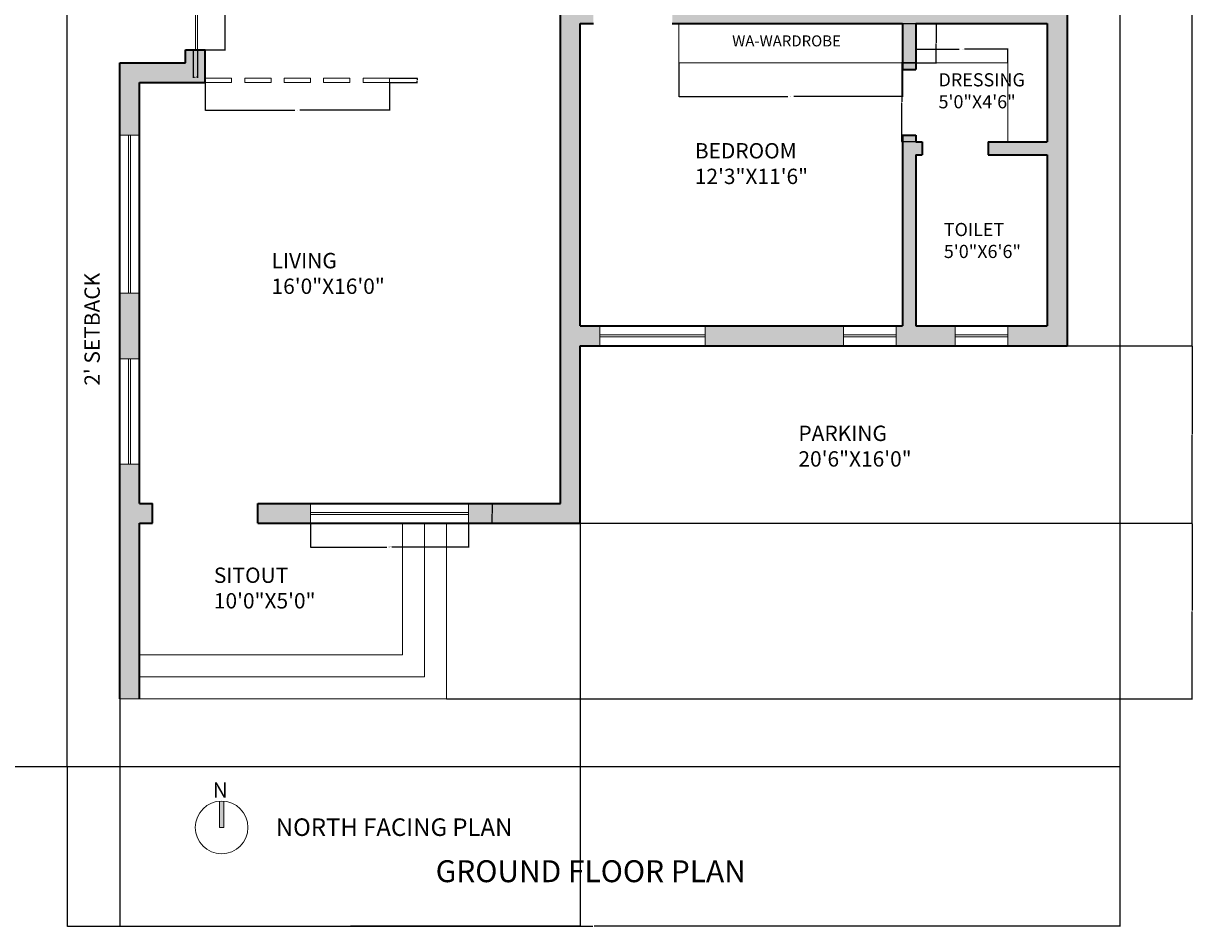
# Model space of a CAD drawing. Units: inches. Extents: x 3386 to 4477, y 1118 to 1824.
# Tile 6 of 7: x 3944 to 4477, y 1118 to 1530. Entities that reach past the tile are written whole.
import ezdxf

# ---------------------------------------------------------------- set-up
doc = ezdxf.new("R2010")
doc.units = ezdxf.units.IN
for name, color, linetype, lineweight in [('A-ANNO-DIMS', 2, 'Continuous', 18), ('A-ANNO-SYMB', 7, 'Continuous', 18), ('A-ANNO-TEXT', 7, 'Continuous', 18), ('A-ANNO-TITL', 7, 'Continuous', 25), ('A-AREA-IDEN', 7, 'Continuous', 18), ('A-DOOR', 4, 'Continuous', 18), ('A-FLOR-CASE', 7, 'Continuous', 18), ('A-FLOR-SCRN', 7, 'Continuous', 18), ('A-FLOR-STRS', 7, 'Continuous', 18), ('A-GLAZ', 4, 'Continuous', 18), ('A-WALL', 7, 'Continuous', 35), ('C-PROP', 7, 'Continuous', 25)]:
    doc.layers.add(name, color=color, linetype=linetype, lineweight=lineweight)
doc.layers.add('A-WALL-PATT', color=18, linetype='Continuous', lineweight=13, true_color=0x000000)
doc.styles.get("Standard").update_dxf_attribs({"font": 'arial.ttf'})
doc.dimstyles.get("Standard").update_dxf_attribs({"dimtxt": 0.18, "dimasz": 0.18, "dimexe": 0.18, "dimexo": 0.0625, "dimgap": 0.09, "dimtad": 0, "dimtih": 1, "dimtoh": 1, "dimdec": 4, "dimzin": 0, "dimdsep": 46, "dimtxsty": 'Standard', "dimcen": 0.09, "dimadec": 0, "dimazin": 0, "dimtfac": 1, "dimtdec": 4, "dimtofl": 0, "dimtmove": 0, "dimatfit": 3, "dimfxl": 1, "dimtolj": 1, "dimtzin": 0, "dimarcsym": 0})

# ---------------------------------------------------------------- blocks, each defined once
blk = doc.blocks.new('WIN-24IN')
for p, q in [((0, 0), (0, 9)), ((24, 0), (24, 9)), ((0, 5), (24, 5)), ((0, 4), (24, 4))]:
    blk.add_line(p, q)
blk = doc.blocks.new('WIN-48IN')
for p, q in [((0, 48), (9, 48)), ((4, 0), (4, 48)), ((5, 0), (5, 48)), ((0, 0), (9, 0))]:
    blk.add_line(p, q)
blk = doc.blocks.new('WIN-72IN')
for p, q in [((0, 0), (0, 9)), ((72, 0), (72, 9)), ((0, 5), (72, 5)), ((0, 4), (72, 4))]:
    blk.add_line(p, q)
blk = doc.blocks.new('DOOR-SLIDING-84IN')
for p, q in [((0, 42), (0, 84)), ((1, 84), (1, 0)), ((1, 42), (0, 42)), ((1, 42), (2, 42)), ((2, 42), (2, 0))]:
    blk.add_line(p, q)
blk = doc.blocks.new('NORTH-ARROW')
at = {"transparency": 33554687}
h = blk.add_hatch(color=256, dxfattribs=at)
h.dxf.hatch_style = 1
h.paths.add_polyline_path([(1, 0), (-1, 0), (-1, 11.96, -0.020861), (0, 12, -0.020861), (1, 11.96)])
for p, q in [((-1, 12), (-1, 0)), ((1, 0), (1, 11.96)), ((-1, 0), (1, 0))]:
    blk.add_line(p, q)
blk.add_circle((0, 0), 12)
blk.add_text('N', height=6.9).set_placement((-4.02, 13.6))
blk = doc.blocks.new('SCREEN-LIVING-DINING')
for points in [[(0, 0), (12, 0), (12, 2), (0, 2)], [(18, 0), (30, 0), (30, 2), (18, 2)], [(36, 0), (48, 0), (48, 2), (36, 2)], [(54, 0), (66, 0), (66, 2), (54, 2)], [(72, 0), (84, 0), (84, 2), (72, 2)]]:
    blk.add_lwpolyline(points, close=True)
blk = doc.blocks.new('WARDROBE-102IN')
for q in [(0, 18), (102, 0)]:
    blk.add_line((0, 0), q)
blk = doc.blocks.new('DRESSING-UNIT-42X36')
for p, q in [((0, 36), (42, 36)), ((42, 36), (42, 0))]:
    blk.add_line(p, q)
blk = doc.blocks.new('*D47')
at = {"layer": 'A-ANNO-DIMS', "color": 0, "lineweight": -2, "transparency": 16777216}
for p, q in [((4074.71, 1301.81), (4074.71, 1290.89)), ((4146.71, 1301.81), (4146.71, 1290.89)), ((4074.89, 1291.07), (4109.59, 1291.07)), ((4146.53, 1291.07), (4111.83, 1291.07))]:
    blk.add_line(p, q, dxfattribs=at)
at = {"layer": 'A-ANNO-DIMS', "color": 0, "transparency": 16777216}
for points in [[(4074.89, 1291.1), (4074.89, 1291.04), (4074.71, 1291.07)], [(4146.53, 1291.1), (4146.53, 1291.04), (4146.71, 1291.07)]]:
    blk.add_solid(points, dxfattribs=at)
at = {"layer": 'Defpoints', "color": 0, "transparency": 16777216}
for p in [(4074.71, 1301.87), (4146.71, 1301.87), (4146.71, 1291.07)]:
    blk.add_point(p, dxfattribs=at)
at = {"layer": 'A-ANNO-DIMS', "color": 0, "transparency": 16777216, "insert": (4110.71, 1291.07), "char_height": 0.18, "attachment_point": 5}
blk.add_mtext('\\A1;WINDOW 72 TYP.', dxfattribs=at)
blk = doc.blocks.new('*D48')
at = {"layer": 'A-ANNO-DIMS', "color": 0, "lineweight": -2, "transparency": 16777216}
for p, q in [((4146.77, 1310.87), (4157.69, 1310.87)), ((4157.51, 1310.69), (4157.51, 1306.55)), ((4146.77, 1301.87), (4157.69, 1301.87)), ((4157.51, 1302.05), (4157.51, 1306.19))]:
    blk.add_line(p, q, dxfattribs=at)
at = {"layer": 'A-ANNO-DIMS', "color": 0, "transparency": 16777216}
for points in [[(4157.48, 1310.69), (4157.54, 1310.69), (4157.51, 1310.87)], [(4157.48, 1302.05), (4157.54, 1302.05), (4157.51, 1301.87)]]:
    blk.add_solid(points, dxfattribs=at)
at = {"layer": 'Defpoints', "color": 0, "transparency": 16777216}
for p in [(4146.71, 1310.87), (4157.51, 1310.87), (4146.71, 1301.87)]:
    blk.add_point(p, dxfattribs=at)
at = {"layer": 'A-ANNO-DIMS', "color": 0, "transparency": 16777216, "insert": (4157.51, 1306.37), "char_height": 0.18, "attachment_point": 5}
blk.add_mtext('\\A1;9 TYP.', dxfattribs=at)
blk = doc.blocks.new('*D51')
at = {"layer": 'A-ANNO-DIMS', "color": 0, "lineweight": -2, "transparency": 16777216}
for p, q in [((4023.27, 1601.87), (4035.99, 1601.87)), ((4035.81, 1601.69), (4035.81, 1560.05)), ((4035.81, 1518.05), (4035.81, 1559.68)), ((4023.27, 1517.87), (4035.99, 1517.87))]:
    blk.add_line(p, q, dxfattribs=at)
at = {"layer": 'A-ANNO-DIMS', "color": 0, "transparency": 16777216}
for points in [[(4035.78, 1601.69), (4035.84, 1601.69), (4035.81, 1601.87)], [(4035.78, 1518.05), (4035.84, 1518.05), (4035.81, 1517.87)]]:
    blk.add_solid(points, dxfattribs=at)
at = {"layer": 'Defpoints', "color": 0, "transparency": 16777216}
for p in [(4023.21, 1601.87), (4023.21, 1517.87), (4035.81, 1517.87)]:
    blk.add_point(p, dxfattribs=at)
at = {"layer": 'A-ANNO-DIMS', "color": 0, "transparency": 16777216, "insert": (4035.81, 1559.87), "char_height": 0.18, "attachment_point": 5}
blk.add_mtext('\\A1;SLIDER 84 TYP.', dxfattribs=at)
blk = doc.blocks.new('*D52')
at = {"layer": 'A-ANNO-DIMS', "color": 0, "lineweight": -2, "transparency": 16777216}
for p, q in [((4021.21, 1517.81), (4021.21, 1505.09)), ((4023.21, 1517.81), (4023.21, 1505.09)), ((4021.39, 1505.27), (4021.75, 1505.27)), ((4023.03, 1505.27), (4022.67, 1505.27))]:
    blk.add_line(p, q, dxfattribs=at)
at = {"layer": 'A-ANNO-DIMS', "color": 0, "transparency": 16777216}
for points in [[(4021.39, 1505.3), (4021.39, 1505.24), (4021.21, 1505.27)], [(4023.03, 1505.3), (4023.03, 1505.24), (4023.21, 1505.27)]]:
    blk.add_solid(points, dxfattribs=at)
at = {"layer": 'Defpoints', "color": 0, "transparency": 16777216}
for p in [(4021.21, 1517.87), (4023.21, 1517.87), (4021.21, 1505.27)]:
    blk.add_point(p, dxfattribs=at)
at = {"layer": 'A-ANNO-DIMS', "color": 0, "transparency": 16777216, "insert": (4022.21, 1505.27), "char_height": 0.18, "attachment_point": 5}
blk.add_mtext('\\A1;2 TYP.', dxfattribs=at)
blk = doc.blocks.new('*D53')
at = {"layer": 'A-ANNO-DIMS', "color": 0, "lineweight": -2, "transparency": 16777216}
for p, q in [((4026.71, 1502.81), (4026.71, 1490.09)), ((4110.71, 1502.81), (4110.71, 1490.09)), ((4026.89, 1490.27), (4067.62, 1490.27)), ((4110.53, 1490.27), (4069.8, 1490.27))]:
    blk.add_line(p, q, dxfattribs=at)
at = {"layer": 'A-ANNO-DIMS', "color": 0, "transparency": 16777216}
for points in [[(4026.89, 1490.3), (4026.89, 1490.24), (4026.71, 1490.27)], [(4110.53, 1490.3), (4110.53, 1490.24), (4110.71, 1490.27)]]:
    blk.add_solid(points, dxfattribs=at)
at = {"layer": 'Defpoints', "color": 0, "transparency": 16777216}
for p in [(4026.71, 1502.87), (4110.71, 1502.87), (4110.71, 1490.27)]:
    blk.add_point(p, dxfattribs=at)
at = {"layer": 'A-ANNO-DIMS', "color": 0, "transparency": 16777216, "insert": (4068.71, 1490.27), "char_height": 0.18, "attachment_point": 5}
blk.add_mtext('\\A1;SCREEN 84 TYP.', dxfattribs=at)
blk = doc.blocks.new('*D54')
at = {"layer": 'A-ANNO-DIMS', "color": 0, "lineweight": -2, "transparency": 16777216}
for p, q in [((4110.77, 1504.87), (4123.49, 1504.87)), ((4123.31, 1504.69), (4123.31, 1504.05)), ((4123.31, 1503.05), (4123.31, 1503.69)), ((4110.77, 1502.87), (4123.49, 1502.87))]:
    blk.add_line(p, q, dxfattribs=at)
at = {"layer": 'A-ANNO-DIMS', "color": 0, "transparency": 16777216}
for points in [[(4123.28, 1504.69), (4123.34, 1504.69), (4123.31, 1504.87)], [(4123.28, 1503.05), (4123.34, 1503.05), (4123.31, 1502.87)]]:
    blk.add_solid(points, dxfattribs=at)
at = {"layer": 'Defpoints', "color": 0, "transparency": 16777216}
for p in [(4110.71, 1504.87), (4123.31, 1504.87), (4110.71, 1502.87)]:
    blk.add_point(p, dxfattribs=at)
at = {"layer": 'A-ANNO-DIMS', "color": 0, "transparency": 16777216, "insert": (4123.31, 1503.87), "char_height": 0.18, "attachment_point": 5}
blk.add_mtext('\\A1;2 TYP.', dxfattribs=at)
blk = doc.blocks.new('*D55')
at = {"layer": 'A-ANNO-DIMS', "color": 0, "lineweight": -2, "transparency": 16777216}
for p, q in [((4242.71, 1511.81), (4242.71, 1496.39)), ((4344.71, 1511.81), (4344.71, 1496.39)), ((4242.89, 1496.57), (4292.33, 1496.57)), ((4344.53, 1496.57), (4295.09, 1496.57))]:
    blk.add_line(p, q, dxfattribs=at)
at = {"layer": 'A-ANNO-DIMS', "color": 0, "transparency": 16777216}
for points in [[(4242.89, 1496.6), (4242.89, 1496.54), (4242.71, 1496.57)], [(4344.53, 1496.6), (4344.53, 1496.54), (4344.71, 1496.57)]]:
    blk.add_solid(points, dxfattribs=at)
at = {"layer": 'Defpoints', "color": 0, "transparency": 16777216}
for p in [(4242.71, 1511.87), (4344.71, 1511.87), (4344.71, 1496.57)]:
    blk.add_point(p, dxfattribs=at)
at = {"layer": 'A-ANNO-DIMS', "color": 0, "transparency": 16777216, "insert": (4293.71, 1496.57), "char_height": 0.18, "attachment_point": 5}
blk.add_mtext('\\A1;WARDROBE 102 TYP.', dxfattribs=at)
blk = doc.blocks.new('*D56')
at = {"layer": 'A-ANNO-DIMS', "color": 0, "lineweight": -2, "transparency": 16777216}
for p, q in [((4344.77, 1529.87), (4360.19, 1529.87)), ((4360.01, 1529.69), (4360.01, 1521.05)), ((4360.01, 1512.05), (4360.01, 1520.69)), ((4344.77, 1511.87), (4360.19, 1511.87))]:
    blk.add_line(p, q, dxfattribs=at)
at = {"layer": 'A-ANNO-DIMS', "color": 0, "transparency": 16777216}
for points in [[(4359.98, 1529.69), (4360.04, 1529.69), (4360.01, 1529.87)], [(4359.98, 1512.05), (4360.04, 1512.05), (4360.01, 1511.87)]]:
    blk.add_solid(points, dxfattribs=at)
at = {"layer": 'Defpoints', "color": 0, "transparency": 16777216}
for p in [(4344.71, 1529.87), (4360.01, 1529.87), (4344.71, 1511.87)]:
    blk.add_point(p, dxfattribs=at)
at = {"layer": 'A-ANNO-DIMS', "color": 0, "transparency": 16777216, "insert": (4360.01, 1520.87), "char_height": 0.18, "attachment_point": 5}
blk.add_mtext('\\A1;18 TYP.', dxfattribs=at)
blk = doc.blocks.new('*D61')
at = {"layer": 'A-ANNO-DIMS', "color": 0, "lineweight": -2, "transparency": 16777216}
for p, q in [((4350.71, 1511.93), (4350.71, 1518.35)), ((4350.89, 1518.17), (4370.54, 1518.17)), ((4392.53, 1518.17), (4372.88, 1518.17)), ((4392.71, 1511.93), (4392.71, 1518.35))]:
    blk.add_line(p, q, dxfattribs=at)
at = {"layer": 'A-ANNO-DIMS', "color": 0, "transparency": 16777216}
for points in [[(4350.89, 1518.2), (4350.89, 1518.14), (4350.71, 1518.17)], [(4392.53, 1518.2), (4392.53, 1518.14), (4392.71, 1518.17)]]:
    blk.add_solid(points, dxfattribs=at)
at = {"layer": 'Defpoints', "color": 0, "transparency": 16777216}
for p in [(4392.71, 1518.17), (4350.71, 1511.87), (4392.71, 1511.87)]:
    blk.add_point(p, dxfattribs=at)
at = {"layer": 'A-ANNO-DIMS', "color": 0, "transparency": 16777216, "insert": (4371.71, 1518.17), "char_height": 0.18, "attachment_point": 5}
blk.add_mtext('\\A1;DRESSER 42 TYP.', dxfattribs=at)
blk = doc.blocks.new('*D62')
at = {"layer": 'A-ANNO-DIMS', "color": 0, "lineweight": -2, "transparency": 16777216}
for p, q in [((4350.65, 1511.87), (4344.23, 1511.87)), ((4344.41, 1511.69), (4344.41, 1494.05)), ((4344.41, 1476.05), (4344.41, 1493.69)), ((4350.65, 1475.87), (4344.23, 1475.87))]:
    blk.add_line(p, q, dxfattribs=at)
at = {"layer": 'A-ANNO-DIMS', "color": 0, "transparency": 16777216}
for points in [[(4344.38, 1511.69), (4344.44, 1511.69), (4344.41, 1511.87)], [(4344.38, 1476.05), (4344.44, 1476.05), (4344.41, 1475.87)]]:
    blk.add_solid(points, dxfattribs=at)
at = {"layer": 'Defpoints', "color": 0, "transparency": 16777216}
for p in [(4344.41, 1511.87), (4350.71, 1511.87), (4350.71, 1475.87)]:
    blk.add_point(p, dxfattribs=at)
at = {"layer": 'A-ANNO-DIMS', "color": 0, "transparency": 16777216, "insert": (4344.41, 1493.87), "char_height": 0.18, "attachment_point": 5}
blk.add_mtext('\\A1;36 TYP.', dxfattribs=at)
blk = doc.blocks.new('*D105')
at = {"layer": 'A-ANNO-DIMS', "color": 0, "lineweight": -2, "transparency": 16777216}
for p, q in [((3963.71, 1190.81), (3963.71, 1117.96)), ((4443.71, 1190.81), (4443.71, 1117.96)), ((3963.89, 1118.14), (4203.42, 1118.14)), ((4443.53, 1118.14), (4204, 1118.14))]:
    blk.add_line(p, q, dxfattribs=at)
at = {"layer": 'A-ANNO-DIMS', "color": 0, "transparency": 16777216}
for points in [[(3963.89, 1118.17), (3963.89, 1118.11), (3963.71, 1118.14)], [(4443.53, 1118.17), (4443.53, 1118.11), (4443.71, 1118.14)]]:
    blk.add_solid(points, dxfattribs=at)
at = {"layer": 'Defpoints', "color": 0, "transparency": 16777216}
for p in [(3963.71, 1190.87), (4443.71, 1190.87), (4443.71, 1118.14)]:
    blk.add_point(p, dxfattribs=at)
at = {"layer": 'A-ANNO-DIMS', "color": 0, "transparency": 16777216, "insert": (4203.71, 1118.14), "char_height": 0.18, "attachment_point": 5}
blk.add_mtext('\\A1;480', dxfattribs=at)
blk = doc.blocks.new('*D106')
at = {"layer": 'A-ANNO-DIMS', "color": 0, "lineweight": -2, "transparency": 16777216}
for p, q in [((3963.65, 1790.87), (3930.48, 1790.87)), ((3930.66, 1790.69), (3930.66, 1491.05)), ((3930.66, 1191.05), (3930.66, 1490.69)), ((3963.65, 1190.87), (3930.48, 1190.87))]:
    blk.add_line(p, q, dxfattribs=at)
at = {"layer": 'A-ANNO-DIMS', "color": 0, "transparency": 16777216}
for points in [[(3930.63, 1790.69), (3930.69, 1790.69), (3930.66, 1790.87)], [(3930.63, 1191.05), (3930.69, 1191.05), (3930.66, 1190.87)]]:
    blk.add_solid(points, dxfattribs=at)
at = {"layer": 'Defpoints', "color": 0, "transparency": 16777216}
for p in [(3930.66, 1790.87), (3963.71, 1790.87), (3963.71, 1190.87)]:
    blk.add_point(p, dxfattribs=at)
at = {"layer": 'A-ANNO-DIMS', "color": 0, "transparency": 16777216, "insert": (3930.66, 1490.87), "char_height": 0.18, "attachment_point": 5}
blk.add_mtext('\\A1;600', dxfattribs=at)
blk = doc.blocks.new('*D108')
at = {"layer": 'A-ANNO-DIMS', "color": 0, "lineweight": -2, "transparency": 16777216}
for p, q in [((4197.71, 1301.81), (4197.71, 1117.96)), ((3987.71, 1221.81), (3987.71, 1117.96)), ((3987.89, 1118.14), (4092.42, 1118.14)), ((4197.53, 1118.14), (4093, 1118.14))]:
    blk.add_line(p, q, dxfattribs=at)
at = {"layer": 'A-ANNO-DIMS', "color": 0, "transparency": 16777216}
for points in [[(3987.89, 1118.17), (3987.89, 1118.11), (3987.71, 1118.14)], [(4197.53, 1118.17), (4197.53, 1118.11), (4197.71, 1118.14)]]:
    blk.add_solid(points, dxfattribs=at)
at = {"layer": 'Defpoints', "color": 0, "transparency": 16777216}
for p in [(4197.71, 1301.87), (3987.71, 1221.87), (4197.71, 1118.14)]:
    blk.add_point(p, dxfattribs=at)
at = {"layer": 'A-ANNO-DIMS', "color": 0, "transparency": 16777216, "insert": (4092.71, 1118.14), "char_height": 0.18, "attachment_point": 5}
blk.add_mtext('\\A1;210', dxfattribs=at)
blk = doc.blocks.new('*D109')
at = {"layer": 'A-ANNO-DIMS', "color": 0, "lineweight": -2, "transparency": 16777216}
for p, q in [((4197.77, 1301.87), (4476.94, 1301.87)), ((4476.76, 1301.69), (4476.76, 1262.05)), ((4476.76, 1222.05), (4476.76, 1261.69)), ((4136.77, 1221.87), (4476.94, 1221.87))]:
    blk.add_line(p, q, dxfattribs=at)
at = {"layer": 'A-ANNO-DIMS', "color": 0, "transparency": 16777216}
for points in [[(4476.73, 1301.69), (4476.79, 1301.69), (4476.76, 1301.87)], [(4476.73, 1222.05), (4476.79, 1222.05), (4476.76, 1221.87)]]:
    blk.add_solid(points, dxfattribs=at)
at = {"layer": 'Defpoints', "color": 0, "transparency": 16777216}
for p in [(4197.71, 1301.87), (4476.76, 1301.87), (4136.71, 1221.87)]:
    blk.add_point(p, dxfattribs=at)
at = {"layer": 'A-ANNO-DIMS', "color": 0, "transparency": 16777216, "insert": (4476.76, 1261.87), "char_height": 0.18, "attachment_point": 5}
blk.add_mtext('\\A1;80', dxfattribs=at)
blk = doc.blocks.new('*D110')
at = {"layer": 'A-ANNO-DIMS', "color": 0, "lineweight": -2, "transparency": 16777216}
for p, q in [((4419.77, 1382.87), (4476.94, 1382.87)), ((4476.76, 1382.69), (4476.76, 1342.55)), ((4476.76, 1302.05), (4476.76, 1342.19)), ((4197.77, 1301.87), (4476.94, 1301.87))]:
    blk.add_line(p, q, dxfattribs=at)
at = {"layer": 'A-ANNO-DIMS', "color": 0, "transparency": 16777216}
for points in [[(4476.73, 1382.69), (4476.79, 1382.69), (4476.76, 1382.87)], [(4476.73, 1302.05), (4476.79, 1302.05), (4476.76, 1301.87)]]:
    blk.add_solid(points, dxfattribs=at)
at = {"layer": 'Defpoints', "color": 0, "transparency": 16777216}
for p in [(4419.71, 1382.87), (4476.76, 1382.87), (4197.71, 1301.87)]:
    blk.add_point(p, dxfattribs=at)
at = {"layer": 'A-ANNO-DIMS', "color": 0, "transparency": 16777216, "insert": (4476.76, 1342.37), "char_height": 0.18, "attachment_point": 5}
blk.add_mtext('\\A1;81', dxfattribs=at)
blk = doc.blocks.new('*D111')
at = {"layer": 'A-ANNO-DIMS', "color": 0, "lineweight": -2, "transparency": 16777216}
for p, q in [((4419.77, 1766.87), (4476.94, 1766.87)), ((4476.76, 1766.69), (4476.76, 1575.05)), ((4476.76, 1383.05), (4476.76, 1574.69)), ((4419.77, 1382.87), (4476.94, 1382.87))]:
    blk.add_line(p, q, dxfattribs=at)
at = {"layer": 'A-ANNO-DIMS', "color": 0, "transparency": 16777216}
for points in [[(4476.73, 1766.69), (4476.79, 1766.69), (4476.76, 1766.87)], [(4476.73, 1383.05), (4476.79, 1383.05), (4476.76, 1382.87)]]:
    blk.add_solid(points, dxfattribs=at)
at = {"layer": 'Defpoints', "color": 0, "transparency": 16777216}
for p in [(4419.71, 1766.87), (4476.76, 1766.87), (4419.71, 1382.87)]:
    blk.add_point(p, dxfattribs=at)
at = {"layer": 'A-ANNO-DIMS', "color": 0, "transparency": 16777216, "insert": (4476.76, 1574.87), "char_height": 0.18, "attachment_point": 5}
blk.add_mtext('\\A1;384', dxfattribs=at)

msp = doc.modelspace()

# ---------------------------------------------------------------- hatches: boundary and pattern name
at = {"layer": 'A-WALL-PATT'}
h = msp.add_hatch(color=256, dxfattribs=at)
h.dxf.hatch_style = 1
h.paths.add_polyline_path([(4131.71, 1766.87), (4131.71, 1745.87), (4125.71, 1745.87), (4125.71, 1736.87), (4131.71, 1736.87), (4131.71, 1712.87), (4140.71, 1712.87), (4140.71, 1757.87), (4188.71, 1757.87), (4188.71, 1679.87), (4140.71, 1679.87), (4140.71, 1682.87), (4131.71, 1682.87), (4131.71, 1607.87), (4146.71, 1607.87), (4146.71, 1613.87), (4140.71, 1613.87), (4140.71, 1673.87), (4188.71, 1673.87), (4188.71, 1613.87), (4182.71, 1613.87), (4182.71, 1607.87), (4269.71, 1607.87), (4269.71, 1613.87), (4266.71, 1613.87), (4266.71, 1634.87), (4260.71, 1634.87), (4260.71, 1613.87), (4194.71, 1613.87), (4194.71, 1673.87), (4227.71, 1673.87), (4227.71, 1679.87), (4194.71, 1679.87), (4194.71, 1757.87), (4215.71, 1757.87), (4215.71, 1766.87)])
h.paths.add_polyline_path([(3987.71, 1688.87), (3996.71, 1688.87), (3996.71, 1736.87), (4035.71, 1736.87), (4035.71, 1745.87), (3987.71, 1745.87)])
h.paths.add_polyline_path([(3996.71, 1616.87), (3996.71, 1640.87), (3987.71, 1640.87), (3987.71, 1607.87), (4017.71, 1607.87), (4017.71, 1601.87), (4026.71, 1601.87), (4026.71, 1616.87)])
h.paths.add_polyline_path([(3987.71, 1511.87), (3987.71, 1478.87), (3996.71, 1478.87), (3996.71, 1502.87), (4026.71, 1502.87), (4026.71, 1517.87), (4017.71, 1517.87), (4017.71, 1511.87)])
h.paths.add_polyline_path([(3996.71, 1406.87), (3987.71, 1406.87), (3987.71, 1376.87), (3996.71, 1376.87)])
h.paths.add_polyline_path([(3996.71, 1310.87), (3996.71, 1328.87), (3987.71, 1328.87), (3987.71, 1221.87), (3996.71, 1221.87), (3996.71, 1301.87), (4002.71, 1301.87), (4002.71, 1310.87)])
h.paths.add_polyline_path([(4050.71, 1310.87), (4050.71, 1301.87), (4074.71, 1301.87), (4074.71, 1310.87)])
h.paths.add_polyline_path([(4197.71, 1301.87), (4197.71, 1382.87), (4206.71, 1382.87), (4206.71, 1391.87), (4197.71, 1391.87), (4197.71, 1529.87), (4203.71, 1529.87), (4203.71, 1535.87), (4188.71, 1535.87), (4188.71, 1310.87), (4146.71, 1310.87), (4146.71, 1301.87)])
h.paths.add_polyline_path([(4254.71, 1391.87), (4254.71, 1382.87), (4317.71, 1382.87), (4317.71, 1391.87)], flags=17)
h.paths.add_polyline_path([(4350.71, 1469.87), (4353.71, 1469.87), (4353.71, 1475.87), (4350.71, 1475.87), (4350.71, 1478.87), (4344.71, 1478.87), (4344.71, 1391.87), (4341.71, 1391.87), (4341.71, 1382.87), (4368.71, 1382.87), (4368.71, 1391.87), (4350.71, 1391.87)], flags=17)
h.paths.add_polyline_path([(4419.71, 1547.87), (4410.71, 1547.87), (4410.71, 1535.87), (4239.71, 1535.87), (4239.71, 1529.87), (4344.71, 1529.87), (4344.71, 1508.87), (4350.71, 1508.87), (4350.71, 1529.87), (4410.71, 1529.87), (4410.71, 1475.87), (4383.71, 1475.87), (4383.71, 1469.87), (4410.71, 1469.87), (4410.71, 1391.87), (4392.71, 1391.87), (4392.71, 1382.87), (4419.71, 1382.87)])
h.paths.add_polyline_path([(4419.71, 1673.87), (4410.71, 1673.87), (4410.71, 1613.87), (4305.71, 1613.87), (4305.71, 1607.87), (4410.71, 1607.87), (4410.71, 1595.87), (4419.71, 1595.87)])
h.paths.add_polyline_path([(4410.71, 1733.87), (4419.71, 1733.87), (4419.71, 1766.87), (4398.71, 1766.87), (4398.71, 1757.87), (4410.71, 1757.87)])
h.paths.add_polyline_path([(4266.71, 1757.87), (4272.71, 1757.87), (4272.71, 1766.87), (4239.71, 1766.87), (4239.71, 1757.87), (4260.71, 1757.87), (4260.71, 1679.87), (4257.71, 1679.87), (4257.71, 1673.87), (4260.71, 1673.87), (4260.71, 1664.87), (4266.71, 1664.87)])
h.paths.add_polyline_path([(4350.71, 1757.87), (4350.71, 1766.87), (4320.71, 1766.87), (4320.71, 1757.87)])
h.paths.add_polyline_path([(4083.71, 1745.87), (4083.71, 1736.87), (4095.71, 1736.87), (4095.71, 1745.87)])

# ---------------------------------------------------------------- linework, layer by layer
at = {"layer": 'A-FLOR-STRS'}
for p, q in [((4116.71, 1241.87), (4116.71, 1301.87)), ((4126.71, 1231.87), (4126.71, 1301.87)), ((4136.71, 1221.87), (4136.71, 1301.87)), ((3996.71, 1241.87), (4116.71, 1241.87)), ((3996.71, 1231.87), (4126.71, 1231.87)), ((3987.71, 1221.87), (4136.71, 1221.87))]:
    msp.add_line(p, q, dxfattribs=at)
at = {"layer": 'A-WALL'}
for p, q in [((4419.71, 1766.87), (4419.71, 1382.87)), ((4188.71, 1310.87), (4188.71, 1535.87)), ((4197.71, 1391.87), (4197.71, 1529.87)), ((4197.71, 1529.87), (4203.71, 1529.87)), ((4239.71, 1529.87), (4344.71, 1529.87)), ((4344.71, 1529.87), (4344.71, 1508.87)), ((4350.71, 1529.87), (4350.71, 1508.87)), ((4350.71, 1529.87), (4410.71, 1529.87)), ((4410.71, 1529.87), (4410.71, 1475.87)), ((4017.71, 1511.87), (4017.71, 1517.87)), ((4017.71, 1517.87), (4026.71, 1517.87)), ((4026.71, 1502.87), (4026.71, 1517.87)), ((3987.71, 1221.87), (3987.71, 1511.87)), ((3987.71, 1511.87), (4017.71, 1511.87)), ((4344.71, 1508.87), (4350.71, 1508.87)), ((3996.71, 1502.87), (4026.71, 1502.87)), ((3996.71, 1310.87), (3996.71, 1502.87)), ((4344.71, 1478.87), (4344.71, 1391.87)), ((4344.71, 1478.87), (4350.71, 1478.87)), ((4350.71, 1478.87), (4350.71, 1475.87)), ((4350.71, 1475.87), (4353.71, 1475.87)), ((4353.71, 1475.87), (4353.71, 1469.87)), ((4383.71, 1475.87), (4383.71, 1469.87)), ((4383.71, 1475.87), (4410.71, 1475.87)), ((4350.71, 1469.87), (4350.71, 1391.87)), ((4350.71, 1469.87), (4353.71, 1469.87)), ((4383.71, 1469.87), (4410.71, 1469.87)), ((4410.71, 1469.87), (4410.71, 1391.87)), ((4197.71, 1391.87), (4344.71, 1391.87)), ((4350.71, 1391.87), (4410.71, 1391.87)), ((4197.71, 1301.87), (4197.71, 1382.87)), ((4197.71, 1382.87), (4419.71, 1382.87)), ((3996.71, 1310.87), (4002.71, 1310.87)), ((4002.71, 1301.87), (4002.71, 1310.87)), ((4050.71, 1310.87), (4188.71, 1310.87)), ((4050.71, 1301.87), (4050.71, 1310.87)), ((3996.71, 1301.87), (4002.71, 1301.87)), ((3996.71, 1221.87), (3996.71, 1301.87)), ((4050.71, 1301.87), (4197.71, 1301.87))]:
    msp.add_line(p, q, dxfattribs=at)
at = {"layer": 'C-PROP'}
msp.add_lwpolyline([(3963.71, 1790.87), (4443.71, 1790.87), (4443.71, 1190.87), (3963.71, 1190.87)], close=True, dxfattribs=at)

# ---------------------------------------------------------------- block references
at = {"layer": 'A-ANNO-SYMB'}
msp.add_blockref('NORTH-ARROW', (4034.19, 1163.19), dxfattribs=at)
at = {"layer": 'A-DOOR', "rotation": 180}
msp.add_blockref('DOOR-SLIDING-84IN', (4023.21, 1601.87), dxfattribs=at)
at = {"layer": 'A-FLOR-CASE'}
for name, p in [('WARDROBE-102IN', (4242.71, 1511.87)), ('DRESSING-UNIT-42X36', (4350.71, 1475.87))]:
    msp.add_blockref(name, p, dxfattribs=at)
at = {"layer": 'A-FLOR-SCRN'}
msp.add_blockref('SCREEN-LIVING-DINING', (4026.71, 1502.87), dxfattribs=at)
at = {"layer": 'A-GLAZ'}
for name, p, rotation in [('WIN-72IN', (3987.71, 1478.87), 270.0000000000004), ('WIN-48IN', (4206.71, 1391.87), 269.9999999999996), ('WIN-24IN', (4341.71, 1391.87), 180), ('WIN-48IN', (3996.71, 1376.87), 180)]:
    msp.add_blockref(name, p, dxfattribs=dict(at, rotation=rotation))
for name, p in [('WIN-24IN', (4368.71, 1382.87)), ('WIN-72IN', (4074.71, 1301.87))]:
    msp.add_blockref(name, p, dxfattribs=at)

# ---------------------------------------------------------------- texts
at = {"layer": 'A-ANNO-TEXT', "insert": (4267.01, 1524.38), "char_height": 5, "attachment_point": 1}
msp.add_mtext_dynamic_manual_height_columns('{\\fTimes New Roman|b0|i0|c0|p18;WA-WARDROBE}', width=79.5604, gutter_width=12.5, heights=[0], dxfattribs=at)
at = {"layer": 'A-ANNO-TEXT', "insert": (3971.64, 1364.63), "char_height": 7, "attachment_point": 1, "rotation": 90}
msp.add_mtext_dynamic_manual_height_columns("{\\fTimes New Roman|b0|i0|c0|p18;2' SETBACK}", width=79.5604, gutter_width=12.5, heights=[0], dxfattribs=at)
at = {"layer": 'A-ANNO-TITL', "attachment_point": 1}
for s, insert, char_height in [('{\\fTimes New Roman|b0|i0|c0|p18;NORTH FACING PLAN}', (4058.88, 1167.31), 8), ('{\\fTimes New Roman|b0|i0|c0|p18;GROUND FLOOR PLAN}', (4131.79, 1148.22), 10)]:
    msp.add_mtext_dynamic_manual_height_columns(s, width=196.2607, gutter_width=12.5, heights=[0], dxfattribs=dict(at, insert=insert, char_height=char_height))
at = {"layer": 'A-AREA-IDEN', "attachment_point": 1}
for s, insert, char_height in [('{\\fTimes New Roman|b0|i0|c0|p18;DRESSING\\P5\'0"X4\'6"}', (4361.1, 1507.13), 6), ('{\\fTimes New Roman|b0|i0|c0|p18;BEDROOM\\P12\'3"X11\'6"}', (4249.97, 1475.27), 7), ('{\\fTimes New Roman|b0|i0|c0|p18;TOILET\\P5\'0"X6\'6"}', (4363.52, 1438.86), 6), ('{\\fTimes New Roman|b0|i0|c0|p18;LIVING\\P16\'0"X16\'0"}', (4056.95, 1425.17), 7), ('{\\fTimes New Roman|b0|i0|c0|p18;PARKING\\P20\'6"X16\'0"}', (4297.2, 1346.42), 7), ('{\\fTimes New Roman|b0|i0|c0|p18;SITOUT\\P10\'0"X5\'0"}', (4030.66, 1281.71), 7)]:
    msp.add_mtext_dynamic_manual_height_columns(s, width=79.5604, gutter_width=12.5, heights=[0], dxfattribs=dict(at, insert=insert, char_height=char_height))

# ---------------------------------------------------------------- dimensions: what is measured, and where the dimension line sits
at = {"layer": 'A-ANNO-DIMS'}
for base, p1, p2, picture, middle in [((3930.66, 1790.87), (3963.71, 1190.87), (3963.71, 1790.87), '*D106', (3930.66, 1490.87)), ((4476.76, 1766.87), (4419.71, 1382.87), (4419.71, 1766.87), '*D111', (4476.76, 1574.87)), ((4476.76, 1382.87), (4197.71, 1301.87), (4419.71, 1382.87), '*D110', (4476.76, 1342.37)), ((4476.76, 1301.87), (4136.71, 1221.87), (4197.71, 1301.87), '*D109', (4476.76, 1261.87))]:
    dim = msp.add_linear_dim(base=base, p1=p1, p2=p2, angle=90, dimstyle='Standard', override={"dimdec": 0, "dimlfac": 1, "dimrnd": 0, "dimzin": 0, "dimdsep": 46, "dimlunit": 2}, dxfattribs=at)
    dim.commit()
    dim.dimension.update_dxf_attribs({"geometry": picture, "text_midpoint": middle})
for base, p1, p2, angle, text, picture, middle in [((4035.81, 1517.87), (4023.21, 1601.87), (4023.21, 1517.87), 270, 'SLIDER <> TYP.', '*D51', (4035.81, 1559.87)), ((4360.01, 1529.87), (4344.71, 1511.87), (4344.71, 1529.87), 90, '<> TYP.', '*D56', (4360.01, 1520.87)), ((4021.21, 1505.27), (4023.21, 1517.87), (4021.21, 1517.87), 180, '<> TYP.', '*D52', (4022.21, 1505.27)), ((4344.41, 1511.87), (4350.71, 1475.87), (4350.71, 1511.87), 90, '<> TYP.', '*D62', (4344.41, 1493.87)), ((4123.31, 1504.87), (4110.71, 1502.87), (4110.71, 1504.87), 90, '<> TYP.', '*D54', (4123.31, 1503.87)), ((4157.51, 1310.87), (4146.71, 1301.87), (4146.71, 1310.87), 90, '<> TYP.', '*D48', (4157.51, 1306.37))]:
    dim = msp.add_linear_dim(base=base, p1=p1, p2=p2, angle=angle, text=text, dimstyle='Standard', override={"dimdec": 0, "dimlfac": 1, "dimrnd": 0, "dimzin": 0, "dimdsep": 46, "dimlunit": 2}, dxfattribs=at)
    dim.commit()
    dim.dimension.update_dxf_attribs({"geometry": picture, "text_midpoint": middle})
for base, p1, p2, text, picture, middle in [((4392.71, 1518.17), (4350.71, 1511.87), (4392.71, 1511.87), 'DRESSER <> TYP.', '*D61', (4371.71, 1518.17)), ((4344.71, 1496.57), (4242.71, 1511.87), (4344.71, 1511.87), 'WARDROBE <> TYP.', '*D55', (4293.71, 1496.57)), ((4110.71, 1490.27), (4026.71, 1502.87), (4110.71, 1502.87), 'SCREEN <> TYP.', '*D53', (4068.71, 1490.27)), ((4146.71, 1291.07), (4074.71, 1301.87), (4146.71, 1301.87), 'WINDOW <> TYP.', '*D47', (4110.71, 1291.07))]:
    dim = msp.add_linear_dim(base=base, p1=p1, p2=p2, text=text, dimstyle='Standard', override={"dimdec": 0, "dimlfac": 1, "dimrnd": 0, "dimzin": 0, "dimdsep": 46, "dimlunit": 2}, dxfattribs=at)
    dim.commit()
    dim.dimension.update_dxf_attribs({"geometry": picture, "text_midpoint": middle})
for base, p1, p2, picture, middle in [((4197.71, 1118.14), (3987.71, 1221.87), (4197.71, 1301.87), '*D108', (4092.71, 1118.14)), ((4443.71, 1118.14), (3963.71, 1190.87), (4443.71, 1190.87), '*D105', (4203.71, 1118.14))]:
    dim = msp.add_linear_dim(base=base, p1=p1, p2=p2, dimstyle='Standard', override={"dimdec": 0, "dimlfac": 1, "dimrnd": 0, "dimzin": 0, "dimdsep": 46, "dimlunit": 2}, dxfattribs=at)
    dim.commit()
    dim.dimension.update_dxf_attribs({"geometry": picture, "text_midpoint": middle})

doc.saveas('drawing.dxf')
